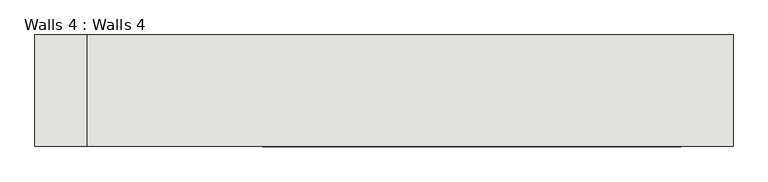
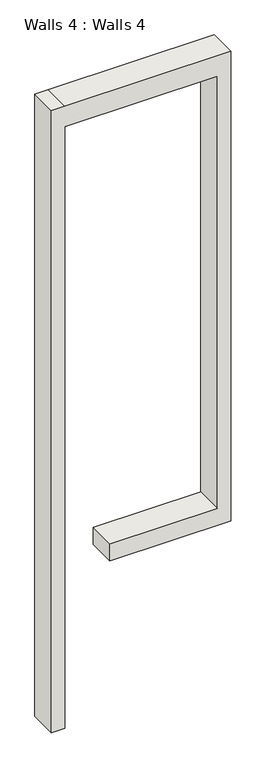
"""IFC4 building model written with IfcOpenShell, lengths in millimetres: wall geometry, Walls 4 : Walls 4."""

from ifc_helpers import new_model, si_unit, frame, origin, place, context, project, spatial, polyline, outline, extrude, source, transform, mapped, element, save


def walls_4_walls_4_370afa2d(model_context):
    return source(origin(), model_context, "Body", "SweptSolid", [
        extrude(outline(polyline([(17278.5126651, -6524.8569651), (6096.0, -6524.8569651), (6096.0, -6296.2569651), (16914.9555037, -6296.2569651), (16914.9555037, -3705.4569651), (9144.0, -3705.4569651), (9144.0, -5530.1462515), (8839.2, -5530.1462515), (8839.2, -3476.8569651), (17278.5126651, -3476.8569651), (17278.5126651, -6296.2569651), (17278.5126651, -6524.8569651)])), frame((0.0, 79.0466379, 0.0), z_axis=(0.0, 1.0, 0.0), x_axis=(0.0, 0.0, 1.0)), (0.0, 0.0, 1.0), 486.7588763),
    ])


if __name__ == "__main__":
    model = new_model("IFC4")
    model_context = context("Model", 3, world=origin())
    ifc_project = project(units=[si_unit("LENGTHUNIT", "METRE", prefix="MILLI")], contexts=[model_context])
    site = spatial("IfcSite", under=ifc_project)
    building = spatial("IfcBuilding", under=site)
    placement = place(None, origin())
    walls_4_walls_4_shape = walls_4_walls_4_370afa2d(model_context)
    element("IfcWall", 1, ObjectType="Walls 4 : Walls 4", at=placement, inside=building, context=model_context, shape_type="MappedRepresentation", body=[
        mapped(walls_4_walls_4_shape, transform((0.0, 0.0, 0.0), x_axis=(1.0, 0.0, 0.0), y_axis=(0.0, 1.0, 0.0), z_axis=(0.0, 0.0, 1.0))),
    ])
    save(model, "model.ifc")

# Revit data of these elements
# Element 1 (IfcWall, "Walls 4 : Walls 4")
#   Materials on its faces: "1 wall brown", "Default Wall"
# Materials
#   "1 wall brown": class "Generic", colour RGB 61 46 37, transparency 0, Cost = 0
#   "Default Wall": colour RGB 128 128 128, transparency 0, Cost = 0
